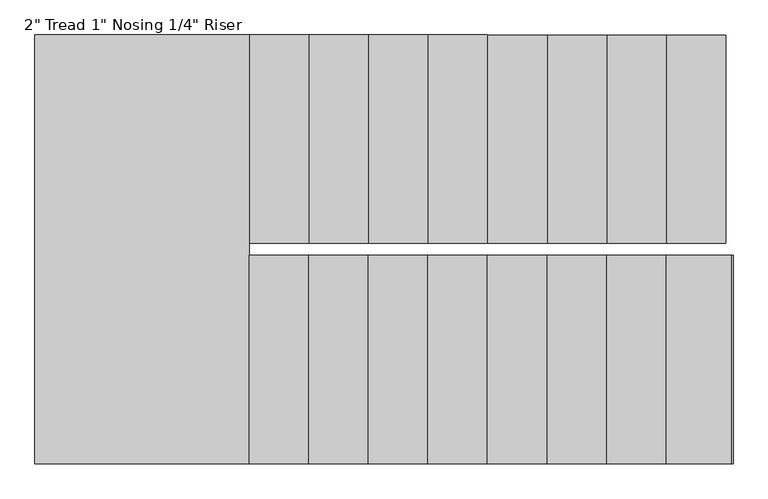
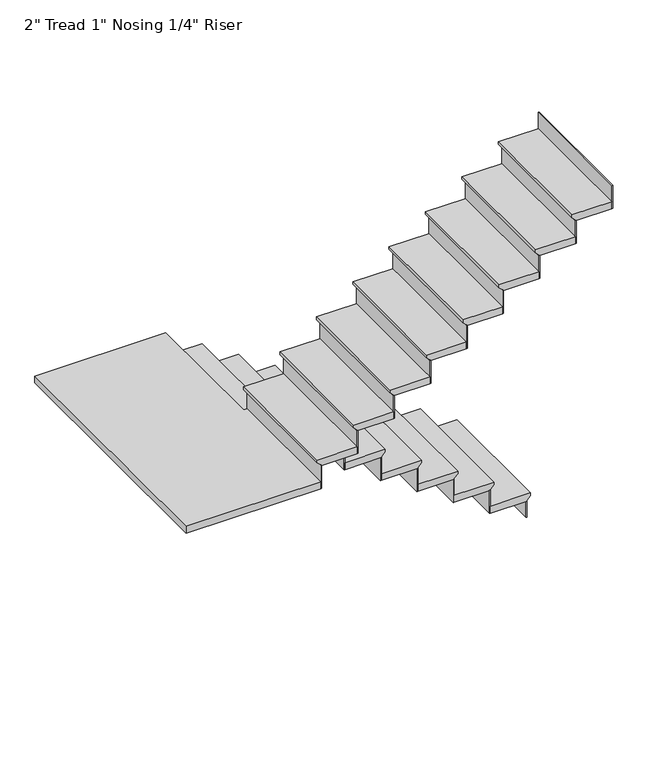
"""IFC4 building model written with IfcOpenShell, lengths in millimetres: stair flight geometry."""

from ifc_helpers import new_model, si_unit, origin, place, context, project, spatial, faceted_brep, source, transform, mapped, element, save


def stair_flight_d3eadeea(model_context):
    return source(origin(), model_context, "Body", "Brep", [
        faceted_brep([(-2748.0012202, 5930.6309003, 12342.2833333), (-2748.0012202, 5930.6309003, 12361.3333333), (-2748.0012202, 5041.6309003, 12361.3333333), (-2748.0012202, 5041.6309003, 12342.2833333), (-2773.4012202, 5930.6309003, 12316.8833333), (-2773.4012202, 5041.6309003, 12316.8833333), (-3027.4012202, 5930.6309003, 12361.3333333), (-3027.4012202, 5041.6309003, 12361.3333333), (-2773.4012202, 5041.6309003, 12310.5333333), (-3027.4012202, 5041.6309003, 12310.5333333), (-3027.4012202, 5930.6309003, 12310.5333333), (-2773.4012202, 5930.6309003, 12310.5333333)], [[[0, 1, 2, 3]], [[4, 0, 3, 5]], [[2, 1, 6, 7]], [[8, 9, 10, 11]], [[2, 7, 9, 8, 5, 3]], [[8, 11, 4, 5]], [[6, 1, 0, 4, 11, 10]], [[7, 6, 10, 9]]]),
        faceted_brep([(-2773.4012202, 5930.6309003, 12310.5333333), (-2773.4012202, 5930.6309003, 12192.0), (-2779.7512202, 5930.6309003, 12192.0), (-2779.7512202, 5930.6309003, 12310.5333333), (-2773.4012202, 5041.6309003, 12310.5333333), (-2779.7512202, 5041.6309003, 12310.5333333), (-2779.7512202, 5041.6309003, 12192.0), (-2773.4012202, 5041.6309003, 12192.0)], [[[0, 1, 2, 3]], [[4, 5, 6, 7]], [[1, 0, 4, 7]], [[2, 1, 7, 6]], [[3, 2, 6, 5]], [[0, 3, 5, 4]]]),
        faceted_brep([(-3027.4012202, 5930.6309003, 12479.8666667), (-3027.4012202, 5930.6309003, 12310.5333333), (-3033.7512202, 5930.6309003, 12310.5333333), (-3033.7512202, 5930.6309003, 12479.8666667), (-3027.4012202, 5041.6309003, 12479.8666667), (-3033.7512202, 5041.6309003, 12479.8666667), (-3033.7512202, 5041.6309003, 12310.5333333), (-3027.4012202, 5041.6309003, 12310.5333333)], [[[0, 1, 2, 3]], [[4, 5, 6, 7]], [[1, 0, 4, 7]], [[2, 1, 7, 6]], [[3, 2, 6, 5]], [[0, 3, 5, 4]]]),
        faceted_brep([(-3002.0012202, 5041.6309003, 12530.6666667), (-3002.0012202, 5930.6309003, 12530.6666667), (-3281.4012202, 5930.6309003, 12530.6666667), (-3281.4012202, 5041.6309003, 12530.6666667), (-3027.4012202, 5041.6309003, 12479.8666667), (-3281.4012202, 5041.6309003, 12479.8666667), (-3281.4012202, 5930.6309003, 12479.8666667), (-3027.4012202, 5930.6309003, 12479.8666667), (-3027.4012202, 5041.6309003, 12486.2166667), (-3002.0012202, 5041.6309003, 12511.6166667), (-3027.4012202, 5930.6309003, 12486.2166667), (-3002.0012202, 5930.6309003, 12511.6166667)], [[[0, 1, 2, 3]], [[4, 5, 6, 7]], [[0, 3, 5, 4, 8, 9]], [[4, 7, 10, 8]], [[2, 1, 11, 10, 7, 6]], [[3, 2, 6, 5]], [[11, 1, 0, 9]], [[10, 11, 9, 8]]]),
        faceted_brep([(-3281.4012202, 5930.6309003, 12649.2), (-3281.4012202, 5930.6309003, 12479.8666667), (-3287.7512202, 5930.6309003, 12479.8666667), (-3287.7512202, 5930.6309003, 12649.2), (-3281.4012202, 5041.6309003, 12649.2), (-3287.7512202, 5041.6309003, 12649.2), (-3287.7512202, 5041.6309003, 12479.8666667), (-3281.4012202, 5041.6309003, 12479.8666667)], [[[0, 1, 2, 3]], [[4, 5, 6, 7]], [[1, 0, 4, 7]], [[2, 1, 7, 6]], [[3, 2, 6, 5]], [[0, 3, 5, 4]]]),
        faceted_brep([(-3256.0012202, 5041.6309003, 12700.0), (-3256.0012202, 5930.6309003, 12700.0), (-3535.4012202, 5930.6309003, 12700.0), (-3535.4012202, 5041.6309003, 12700.0), (-3281.4012202, 5041.6309003, 12649.2), (-3535.4012202, 5041.6309003, 12649.2), (-3535.4012202, 5930.6309003, 12649.2), (-3281.4012202, 5930.6309003, 12649.2), (-3281.4012202, 5041.6309003, 12655.55), (-3256.0012202, 5041.6309003, 12680.95), (-3281.4012202, 5930.6309003, 12655.55), (-3256.0012202, 5930.6309003, 12680.95)], [[[0, 1, 2, 3]], [[4, 5, 6, 7]], [[0, 3, 5, 4, 8, 9]], [[4, 7, 10, 8]], [[2, 1, 11, 10, 7, 6]], [[3, 2, 6, 5]], [[11, 1, 0, 9]], [[10, 11, 9, 8]]]),
        faceted_brep([(-3535.4012202, 5930.6309003, 12818.5333333), (-3535.4012202, 5930.6309003, 12649.2), (-3541.7512202, 5930.6309003, 12649.2), (-3541.7512202, 5930.6309003, 12818.5333333), (-3535.4012202, 5041.6309003, 12818.5333333), (-3541.7512202, 5041.6309003, 12818.5333333), (-3541.7512202, 5041.6309003, 12649.2), (-3535.4012202, 5041.6309003, 12649.2)], [[[0, 1, 2, 3]], [[4, 5, 6, 7]], [[1, 0, 4, 7]], [[2, 1, 7, 6]], [[3, 2, 6, 5]], [[0, 3, 5, 4]]]),
        faceted_brep([(-3510.0012202, 5041.6309003, 12869.3333333), (-3510.0012202, 5930.6309003, 12869.3333333), (-3789.4012202, 5930.6309003, 12869.3333333), (-3789.4012202, 5041.6309003, 12869.3333333), (-3535.4012202, 5041.6309003, 12818.5333333), (-3789.4012202, 5041.6309003, 12818.5333333), (-3789.4012202, 5930.6309003, 12818.5333333), (-3535.4012202, 5930.6309003, 12818.5333333), (-3535.4012202, 5041.6309003, 12824.8833333), (-3510.0012202, 5041.6309003, 12850.2833333), (-3535.4012202, 5930.6309003, 12824.8833333), (-3510.0012202, 5930.6309003, 12850.2833333)], [[[0, 1, 2, 3]], [[4, 5, 6, 7]], [[0, 3, 5, 4, 8, 9]], [[4, 7, 10, 8]], [[2, 1, 11, 10, 7, 6]], [[3, 2, 6, 5]], [[11, 1, 0, 9]], [[10, 11, 9, 8]]]),
        faceted_brep([(-3789.4012202, 5930.6309003, 12987.8666667), (-3789.4012202, 5930.6309003, 12818.5333333), (-3795.7512202, 5930.6309003, 12818.5333333), (-3795.7512202, 5930.6309003, 12987.8666667), (-3789.4012202, 5041.6309003, 12987.8666667), (-3795.7512202, 5041.6309003, 12987.8666667), (-3795.7512202, 5041.6309003, 12818.5333333), (-3789.4012202, 5041.6309003, 12818.5333333)], [[[0, 1, 2, 3]], [[4, 5, 6, 7]], [[1, 0, 4, 7]], [[2, 1, 7, 6]], [[3, 2, 6, 5]], [[0, 3, 5, 4]]]),
        faceted_brep([(-3764.0012202, 5041.6309003, 13038.6666667), (-3764.0012202, 5930.6309003, 13038.6666667), (-4043.4012202, 5930.6309003, 13038.6666667), (-4043.4012202, 5041.6309003, 13038.6666667), (-3789.4012202, 5041.6309003, 12987.8666667), (-4043.4012202, 5041.6309003, 12987.8666667), (-4043.4012202, 5930.6309003, 12987.8666667), (-3789.4012202, 5930.6309003, 12987.8666667), (-3789.4012202, 5041.6309003, 12994.2166667), (-3764.0012202, 5041.6309003, 13019.6166667), (-3789.4012202, 5930.6309003, 12994.2166667), (-3764.0012202, 5930.6309003, 13019.6166667)], [[[0, 1, 2, 3]], [[4, 5, 6, 7]], [[0, 3, 5, 4, 8, 9]], [[4, 7, 10, 8]], [[2, 1, 11, 10, 7, 6]], [[3, 2, 6, 5]], [[11, 1, 0, 9]], [[10, 11, 9, 8]]]),
        faceted_brep([(-4043.4012202, 5930.6309003, 13157.2), (-4043.4012202, 5930.6309003, 12987.8666667), (-4049.7512202, 5930.6309003, 12987.8666667), (-4049.7512202, 5930.6309003, 13157.2), (-4043.4012202, 5041.6309003, 13157.2), (-4049.7512202, 5041.6309003, 13157.2), (-4049.7512202, 5041.6309003, 12987.8666667), (-4043.4012202, 5041.6309003, 12987.8666667)], [[[0, 1, 2, 3]], [[4, 5, 6, 7]], [[1, 0, 4, 7]], [[2, 1, 7, 6]], [[3, 2, 6, 5]], [[0, 3, 5, 4]]]),
        faceted_brep([(-4018.0012202, 5041.6309003, 13208.0), (-4018.0012202, 5930.6309003, 13208.0), (-4297.4012202, 5930.6309003, 13208.0), (-4297.4012202, 5041.6309003, 13208.0), (-4043.4012202, 5041.6309003, 13157.2), (-4297.4012202, 5041.6309003, 13157.2), (-4297.4012202, 5930.6309003, 13157.2), (-4043.4012202, 5930.6309003, 13157.2), (-4043.4012202, 5041.6309003, 13163.55), (-4018.0012202, 5041.6309003, 13188.95), (-4043.4012202, 5930.6309003, 13163.55), (-4018.0012202, 5930.6309003, 13188.95)], [[[0, 1, 2, 3]], [[4, 5, 6, 7]], [[0, 3, 5, 4, 8, 9]], [[4, 7, 10, 8]], [[2, 1, 11, 10, 7, 6]], [[3, 2, 6, 5]], [[11, 1, 0, 9]], [[10, 11, 9, 8]]]),
        faceted_brep([(-4297.4012202, 5930.6309003, 13326.5333333), (-4297.4012202, 5930.6309003, 13157.2), (-4303.7512202, 5930.6309003, 13157.2), (-4303.7512202, 5930.6309003, 13326.5333333), (-4297.4012202, 5041.6309003, 13326.5333333), (-4303.7512202, 5041.6309003, 13326.5333333), (-4303.7512202, 5041.6309003, 13157.2), (-4297.4012202, 5041.6309003, 13157.2)], [[[0, 1, 2, 3]], [[4, 5, 6, 7]], [[1, 0, 4, 7]], [[2, 1, 7, 6]], [[3, 2, 6, 5]], [[0, 3, 5, 4]]]),
        faceted_brep([(-4272.0012202, 5041.6309003, 13377.3333333), (-4272.0012202, 5930.6309003, 13377.3333333), (-4551.4012202, 5930.6309003, 13377.3333333), (-4551.4012202, 5041.6309003, 13377.3333333), (-4297.4012202, 5041.6309003, 13326.5333333), (-4551.4012202, 5041.6309003, 13326.5333333), (-4551.4012202, 5930.6309003, 13326.5333333), (-4297.4012202, 5930.6309003, 13326.5333333), (-4297.4012202, 5041.6309003, 13332.8833333), (-4272.0012202, 5041.6309003, 13358.2833333), (-4297.4012202, 5930.6309003, 13332.8833333), (-4272.0012202, 5930.6309003, 13358.2833333)], [[[0, 1, 2, 3]], [[4, 5, 6, 7]], [[0, 3, 5, 4, 8, 9]], [[4, 7, 10, 8]], [[2, 1, 11, 10, 7, 6]], [[3, 2, 6, 5]], [[11, 1, 0, 9]], [[10, 11, 9, 8]]]),
        faceted_brep([(-4551.4012202, 5930.6309003, 13495.8666667), (-4551.4012202, 5930.6309003, 13326.5333333), (-4557.7512202, 5930.6309003, 13326.5333333), (-4557.7512202, 5930.6309003, 13495.8666667), (-4551.4012202, 5041.6309003, 13495.8666667), (-4557.7512202, 5041.6309003, 13495.8666667), (-4557.7512202, 5041.6309003, 13326.5333333), (-4551.4012202, 5041.6309003, 13326.5333333)], [[[0, 1, 2, 3]], [[4, 5, 6, 7]], [[1, 0, 4, 7]], [[2, 1, 7, 6]], [[3, 2, 6, 5]], [[0, 3, 5, 4]]]),
        faceted_brep([(-4526.0012202, 5041.6309003, 13546.6666667), (-4526.0012202, 5930.6309003, 13546.6666667), (-4805.4012202, 5930.6309003, 13546.6666667), (-4805.4012202, 5041.6309003, 13546.6666667), (-4551.4012202, 5041.6309003, 13495.8666667), (-4805.4012202, 5041.6309003, 13495.8666667), (-4805.4012202, 5930.6309003, 13495.8666667), (-4551.4012202, 5930.6309003, 13495.8666667), (-4551.4012202, 5041.6309003, 13502.2166667), (-4526.0012202, 5041.6309003, 13527.6166667), (-4551.4012202, 5930.6309003, 13502.2166667), (-4526.0012202, 5930.6309003, 13527.6166667)], [[[0, 1, 2, 3]], [[4, 5, 6, 7]], [[0, 3, 5, 4, 8, 9]], [[4, 7, 10, 8]], [[2, 1, 11, 10, 7, 6]], [[3, 2, 6, 5]], [[11, 1, 0, 9]], [[10, 11, 9, 8]]]),
        faceted_brep([(-4805.4012202, 5930.6309003, 13665.2), (-4805.4012202, 5930.6309003, 13495.8666667), (-4811.7512202, 5930.6309003, 13495.8666667), (-4811.7512202, 5930.6309003, 13665.2), (-4805.4012202, 5041.6309003, 13665.2), (-4811.7512202, 5041.6309003, 13665.2), (-4811.7512202, 5041.6309003, 13495.8666667), (-4805.4012202, 5041.6309003, 13495.8666667)], [[[0, 1, 2, 3]], [[4, 5, 6, 7]], [[1, 0, 4, 7]], [[2, 1, 7, 6]], [[3, 2, 6, 5]], [[0, 3, 5, 4]]]),
        faceted_brep([(-4754.6012202, 4990.8309003, 13716.0), (-4780.0012202, 4990.8309003, 13716.0), (-4780.0012202, 5930.6309003, 13716.0), (-5694.4012202, 5930.6309003, 13716.0), (-5694.4012202, 4101.8309003, 13716.0), (-4754.6012202, 4101.8309003, 13716.0), (-4780.0012202, 4990.8309003, 13665.2), (-4754.6012202, 4990.8309003, 13665.2), (-4754.6012202, 4101.8309003, 13665.2), (-5694.4012202, 4101.8309003, 13665.2), (-5694.4012202, 5930.6309003, 13665.2), (-4805.4012202, 5930.6309003, 13665.2), (-4805.4012202, 5041.6309003, 13665.2), (-4780.0012202, 5041.6309003, 13665.2), (-4780.0012202, 5041.6309003, 13696.95), (-4780.0012202, 5930.6309003, 13696.95), (-4805.4012202, 5041.6309003, 13671.55), (-4805.4012202, 5930.6309003, 13671.55)], [[[0, 1, 2, 3, 4, 5]], [[6, 7, 8, 9, 10, 11, 12, 13]], [[1, 0, 7, 6]], [[2, 1, 6, 13, 14, 15]], [[13, 12, 16, 14]], [[12, 11, 17, 16]], [[3, 2, 15, 17, 11, 10]], [[4, 3, 10, 9]], [[5, 4, 9, 8]], [[0, 5, 8, 7]], [[17, 15, 14, 16]]]),
        faceted_brep([(-4754.6012202, 4101.8309003, 13834.5333333), (-4754.6012202, 4101.8309003, 13665.2), (-4748.2512202, 4101.8309003, 13665.2), (-4748.2512202, 4101.8309003, 13834.5333333), (-4754.6012202, 4990.8309003, 13834.5333333), (-4748.2512202, 4990.8309003, 13834.5333333), (-4748.2512202, 4990.8309003, 13665.2), (-4754.6012202, 4990.8309003, 13665.2)], [[[0, 1, 2, 3]], [[4, 5, 6, 7]], [[1, 0, 4, 7]], [[2, 1, 7, 6]], [[3, 2, 6, 5]], [[0, 3, 5, 4]]]),
        faceted_brep([(-4780.0012202, 4990.8309003, 13885.3333333), (-4780.0012202, 4101.8309003, 13885.3333333), (-4500.6012202, 4101.8309003, 13885.3333333), (-4500.6012202, 4990.8309003, 13885.3333333), (-4754.6012202, 4990.8309003, 13834.5333333), (-4500.6012202, 4990.8309003, 13834.5333333), (-4500.6012202, 4101.8309003, 13834.5333333), (-4754.6012202, 4101.8309003, 13834.5333333), (-4754.6012202, 4990.8309003, 13840.8833333), (-4780.0012202, 4990.8309003, 13866.2833333), (-4754.6012202, 4101.8309003, 13840.8833333), (-4780.0012202, 4101.8309003, 13866.2833333)], [[[0, 1, 2, 3]], [[4, 5, 6, 7]], [[0, 3, 5, 4, 8, 9]], [[4, 7, 10, 8]], [[2, 1, 11, 10, 7, 6]], [[3, 2, 6, 5]], [[11, 1, 0, 9]], [[10, 11, 9, 8]]]),
        faceted_brep([(-4500.6012202, 4101.8309003, 14003.8666667), (-4500.6012202, 4101.8309003, 13834.5333333), (-4494.2512202, 4101.8309003, 13834.5333333), (-4494.2512202, 4101.8309003, 14003.8666667), (-4500.6012202, 4990.8309003, 14003.8666667), (-4494.2512202, 4990.8309003, 14003.8666667), (-4494.2512202, 4990.8309003, 13834.5333333), (-4500.6012202, 4990.8309003, 13834.5333333)], [[[0, 1, 2, 3]], [[4, 5, 6, 7]], [[1, 0, 4, 7]], [[2, 1, 7, 6]], [[3, 2, 6, 5]], [[0, 3, 5, 4]]]),
        faceted_brep([(-4526.0012202, 4990.8309003, 14054.6666667), (-4526.0012202, 4101.8309003, 14054.6666667), (-4246.6012202, 4101.8309003, 14054.6666667), (-4246.6012202, 4990.8309003, 14054.6666667), (-4500.6012202, 4990.8309003, 14003.8666667), (-4246.6012202, 4990.8309003, 14003.8666667), (-4246.6012202, 4101.8309003, 14003.8666667), (-4500.6012202, 4101.8309003, 14003.8666667), (-4500.6012202, 4990.8309003, 14010.2166667), (-4526.0012202, 4990.8309003, 14035.6166667), (-4500.6012202, 4101.8309003, 14010.2166667), (-4526.0012202, 4101.8309003, 14035.6166667)], [[[0, 1, 2, 3]], [[4, 5, 6, 7]], [[0, 3, 5, 4, 8, 9]], [[4, 7, 10, 8]], [[2, 1, 11, 10, 7, 6]], [[3, 2, 6, 5]], [[11, 1, 0, 9]], [[10, 11, 9, 8]]]),
        faceted_brep([(-4246.6012202, 4101.8309003, 14173.2), (-4246.6012202, 4101.8309003, 14003.8666667), (-4240.2512202, 4101.8309003, 14003.8666667), (-4240.2512202, 4101.8309003, 14173.2), (-4246.6012202, 4990.8309003, 14173.2), (-4240.2512202, 4990.8309003, 14173.2), (-4240.2512202, 4990.8309003, 14003.8666667), (-4246.6012202, 4990.8309003, 14003.8666667)], [[[0, 1, 2, 3]], [[4, 5, 6, 7]], [[1, 0, 4, 7]], [[2, 1, 7, 6]], [[3, 2, 6, 5]], [[0, 3, 5, 4]]]),
        faceted_brep([(-4272.0012202, 4990.8309003, 14224.0), (-4272.0012202, 4101.8309003, 14224.0), (-3992.6012202, 4101.8309003, 14224.0), (-3992.6012202, 4990.8309003, 14224.0), (-4246.6012202, 4990.8309003, 14173.2), (-3992.6012202, 4990.8309003, 14173.2), (-3992.6012202, 4101.8309003, 14173.2), (-4246.6012202, 4101.8309003, 14173.2), (-4246.6012202, 4990.8309003, 14179.55), (-4272.0012202, 4990.8309003, 14204.95), (-4246.6012202, 4101.8309003, 14179.55), (-4272.0012202, 4101.8309003, 14204.95)], [[[0, 1, 2, 3]], [[4, 5, 6, 7]], [[0, 3, 5, 4, 8, 9]], [[4, 7, 10, 8]], [[2, 1, 11, 10, 7, 6]], [[3, 2, 6, 5]], [[11, 1, 0, 9]], [[10, 11, 9, 8]]]),
        faceted_brep([(-3992.6012202, 4101.8309003, 14342.5333333), (-3992.6012202, 4101.8309003, 14173.2), (-3986.2512202, 4101.8309003, 14173.2), (-3986.2512202, 4101.8309003, 14342.5333333), (-3992.6012202, 4990.8309003, 14342.5333333), (-3986.2512202, 4990.8309003, 14342.5333333), (-3986.2512202, 4990.8309003, 14173.2), (-3992.6012202, 4990.8309003, 14173.2)], [[[0, 1, 2, 3]], [[4, 5, 6, 7]], [[1, 0, 4, 7]], [[2, 1, 7, 6]], [[3, 2, 6, 5]], [[0, 3, 5, 4]]]),
        faceted_brep([(-4018.0012202, 4990.8309003, 14393.3333333), (-4018.0012202, 4101.8309003, 14393.3333333), (-3738.6012202, 4101.8309003, 14393.3333333), (-3738.6012202, 4990.8309003, 14393.3333333), (-3992.6012202, 4990.8309003, 14342.5333333), (-3738.6012202, 4990.8309003, 14342.5333333), (-3738.6012202, 4101.8309003, 14342.5333333), (-3992.6012202, 4101.8309003, 14342.5333333), (-3992.6012202, 4990.8309003, 14348.8833333), (-4018.0012202, 4990.8309003, 14374.2833333), (-3992.6012202, 4101.8309003, 14348.8833333), (-4018.0012202, 4101.8309003, 14374.2833333)], [[[0, 1, 2, 3]], [[4, 5, 6, 7]], [[0, 3, 5, 4, 8, 9]], [[4, 7, 10, 8]], [[2, 1, 11, 10, 7, 6]], [[3, 2, 6, 5]], [[11, 1, 0, 9]], [[10, 11, 9, 8]]]),
        faceted_brep([(-3738.6012202, 4101.8309003, 14511.8666667), (-3738.6012202, 4101.8309003, 14342.5333333), (-3732.2512202, 4101.8309003, 14342.5333333), (-3732.2512202, 4101.8309003, 14511.8666667), (-3738.6012202, 4990.8309003, 14511.8666667), (-3732.2512202, 4990.8309003, 14511.8666667), (-3732.2512202, 4990.8309003, 14342.5333333), (-3738.6012202, 4990.8309003, 14342.5333333)], [[[0, 1, 2, 3]], [[4, 5, 6, 7]], [[1, 0, 4, 7]], [[2, 1, 7, 6]], [[3, 2, 6, 5]], [[0, 3, 5, 4]]]),
        faceted_brep([(-3764.0012202, 4990.8309003, 14562.6666667), (-3764.0012202, 4101.8309003, 14562.6666667), (-3484.6012202, 4101.8309003, 14562.6666667), (-3484.6012202, 4990.8309003, 14562.6666667), (-3738.6012202, 4990.8309003, 14511.8666667), (-3484.6012202, 4990.8309003, 14511.8666667), (-3484.6012202, 4101.8309003, 14511.8666667), (-3738.6012202, 4101.8309003, 14511.8666667), (-3738.6012202, 4990.8309003, 14518.2166667), (-3764.0012202, 4990.8309003, 14543.6166667), (-3738.6012202, 4101.8309003, 14518.2166667), (-3764.0012202, 4101.8309003, 14543.6166667)], [[[0, 1, 2, 3]], [[4, 5, 6, 7]], [[0, 3, 5, 4, 8, 9]], [[4, 7, 10, 8]], [[2, 1, 11, 10, 7, 6]], [[3, 2, 6, 5]], [[11, 1, 0, 9]], [[10, 11, 9, 8]]]),
        faceted_brep([(-3484.6012202, 4101.8309003, 14681.2), (-3484.6012202, 4101.8309003, 14511.8666667), (-3478.2512202, 4101.8309003, 14511.8666667), (-3478.2512202, 4101.8309003, 14681.2), (-3484.6012202, 4990.8309003, 14681.2), (-3478.2512202, 4990.8309003, 14681.2), (-3478.2512202, 4990.8309003, 14511.8666667), (-3484.6012202, 4990.8309003, 14511.8666667)], [[[0, 1, 2, 3]], [[4, 5, 6, 7]], [[1, 0, 4, 7]], [[2, 1, 7, 6]], [[3, 2, 6, 5]], [[0, 3, 5, 4]]]),
        faceted_brep([(-3510.0012202, 4990.8309003, 14732.0), (-3510.0012202, 4101.8309003, 14732.0), (-3230.6012202, 4101.8309003, 14732.0), (-3230.6012202, 4990.8309003, 14732.0), (-3484.6012202, 4990.8309003, 14681.2), (-3230.6012202, 4990.8309003, 14681.2), (-3230.6012202, 4101.8309003, 14681.2), (-3484.6012202, 4101.8309003, 14681.2), (-3484.6012202, 4990.8309003, 14687.55), (-3510.0012202, 4990.8309003, 14712.95), (-3484.6012202, 4101.8309003, 14687.55), (-3510.0012202, 4101.8309003, 14712.95)], [[[0, 1, 2, 3]], [[4, 5, 6, 7]], [[0, 3, 5, 4, 8, 9]], [[4, 7, 10, 8]], [[2, 1, 11, 10, 7, 6]], [[3, 2, 6, 5]], [[11, 1, 0, 9]], [[10, 11, 9, 8]]]),
        faceted_brep([(-3230.6012202, 4101.8309003, 14850.5333333), (-3230.6012202, 4101.8309003, 14681.2), (-3224.2512202, 4101.8309003, 14681.2), (-3224.2512202, 4101.8309003, 14850.5333333), (-3230.6012202, 4990.8309003, 14850.5333333), (-3224.2512202, 4990.8309003, 14850.5333333), (-3224.2512202, 4990.8309003, 14681.2), (-3230.6012202, 4990.8309003, 14681.2)], [[[0, 1, 2, 3]], [[4, 5, 6, 7]], [[1, 0, 4, 7]], [[2, 1, 7, 6]], [[3, 2, 6, 5]], [[0, 3, 5, 4]]]),
        faceted_brep([(-3256.0012202, 4990.8309003, 14901.3333333), (-3256.0012202, 4101.8309003, 14901.3333333), (-2976.6012202, 4101.8309003, 14901.3333333), (-2976.6012202, 4990.8309003, 14901.3333333), (-3230.6012202, 4990.8309003, 14850.5333333), (-2976.6012202, 4990.8309003, 14850.5333333), (-2976.6012202, 4101.8309003, 14850.5333333), (-3230.6012202, 4101.8309003, 14850.5333333), (-3230.6012202, 4990.8309003, 14856.8833333), (-3256.0012202, 4990.8309003, 14882.2833333), (-3230.6012202, 4101.8309003, 14856.8833333), (-3256.0012202, 4101.8309003, 14882.2833333)], [[[0, 1, 2, 3]], [[4, 5, 6, 7]], [[0, 3, 5, 4, 8, 9]], [[4, 7, 10, 8]], [[2, 1, 11, 10, 7, 6]], [[3, 2, 6, 5]], [[11, 1, 0, 9]], [[10, 11, 9, 8]]]),
        faceted_brep([(-2976.6012202, 4101.8309003, 15019.8666667), (-2976.6012202, 4101.8309003, 14850.5333333), (-2970.2512202, 4101.8309003, 14850.5333333), (-2970.2512202, 4101.8309003, 15019.8666667), (-2976.6012202, 4990.8309003, 15019.8666667), (-2970.2512202, 4990.8309003, 15019.8666667), (-2970.2512202, 4990.8309003, 14850.5333333), (-2976.6012202, 4990.8309003, 14850.5333333)], [[[0, 1, 2, 3]], [[4, 5, 6, 7]], [[1, 0, 4, 7]], [[2, 1, 7, 6]], [[3, 2, 6, 5]], [[0, 3, 5, 4]]]),
        faceted_brep([(-2722.6012202, 4101.8309003, 15189.2), (-2722.6012202, 4101.8309003, 15019.8666667), (-2716.2512202, 4101.8309003, 15019.8666667), (-2716.2512202, 4101.8309003, 15189.2), (-2722.6012202, 4990.8309003, 15189.2), (-2716.2512202, 4990.8309003, 15189.2), (-2716.2512202, 4990.8309003, 15019.8666667), (-2722.6012202, 4990.8309003, 15019.8666667)], [[[0, 1, 2, 3]], [[4, 5, 6, 7]], [[1, 0, 4, 7]], [[2, 1, 7, 6]], [[3, 2, 6, 5]], [[0, 3, 5, 4]]]),
        faceted_brep([(-3002.0012202, 4990.8309003, 15070.6666667), (-3002.0012202, 4101.8309003, 15070.6666667), (-2722.6012202, 4101.8309003, 15070.6666667), (-2722.6012202, 4990.8309003, 15070.6666667), (-2976.6012202, 4990.8309003, 15019.8666667), (-2722.6012202, 4990.8309003, 15019.8666667), (-2722.6012202, 4101.8309003, 15019.8666667), (-2976.6012202, 4101.8309003, 15019.8666667), (-2976.6012202, 4990.8309003, 15026.2166667), (-3002.0012202, 4990.8309003, 15051.6166667), (-2976.6012202, 4101.8309003, 15026.2166667), (-3002.0012202, 4101.8309003, 15051.6166667)], [[[0, 1, 2, 3]], [[4, 5, 6, 7]], [[0, 3, 5, 4, 8, 9]], [[4, 7, 10, 8]], [[2, 1, 11, 10, 7, 6]], [[3, 2, 6, 5]], [[11, 1, 0, 9]], [[10, 11, 9, 8]]]),
    ])


if __name__ == "__main__":
    model = new_model("IFC4")
    model_context = context("Model", 3, world=origin())
    ifc_project = project(units=[si_unit("LENGTHUNIT", "METRE", prefix="MILLI")], contexts=[model_context])
    site = spatial("IfcSite", under=ifc_project)
    building = spatial("IfcBuilding", under=site)
    placement = place(None, origin())
    stair_flight_shape = stair_flight_d3eadeea(model_context)
    element("IfcStairFlight", 1, ObjectType="2\" Tread 1\" Nosing 1/4\" Riser", at=placement, inside=building, context=model_context, shape_type="MappedRepresentation", body=[
        mapped(stair_flight_shape, transform((0.0, 0.0, 0.0), x_axis=(1.0, 0.0, 0.0), y_axis=(0.0, 1.0, 0.0), z_axis=(0.0, 0.0, 1.0))),
    ])
    save(model, "model.ifc")
